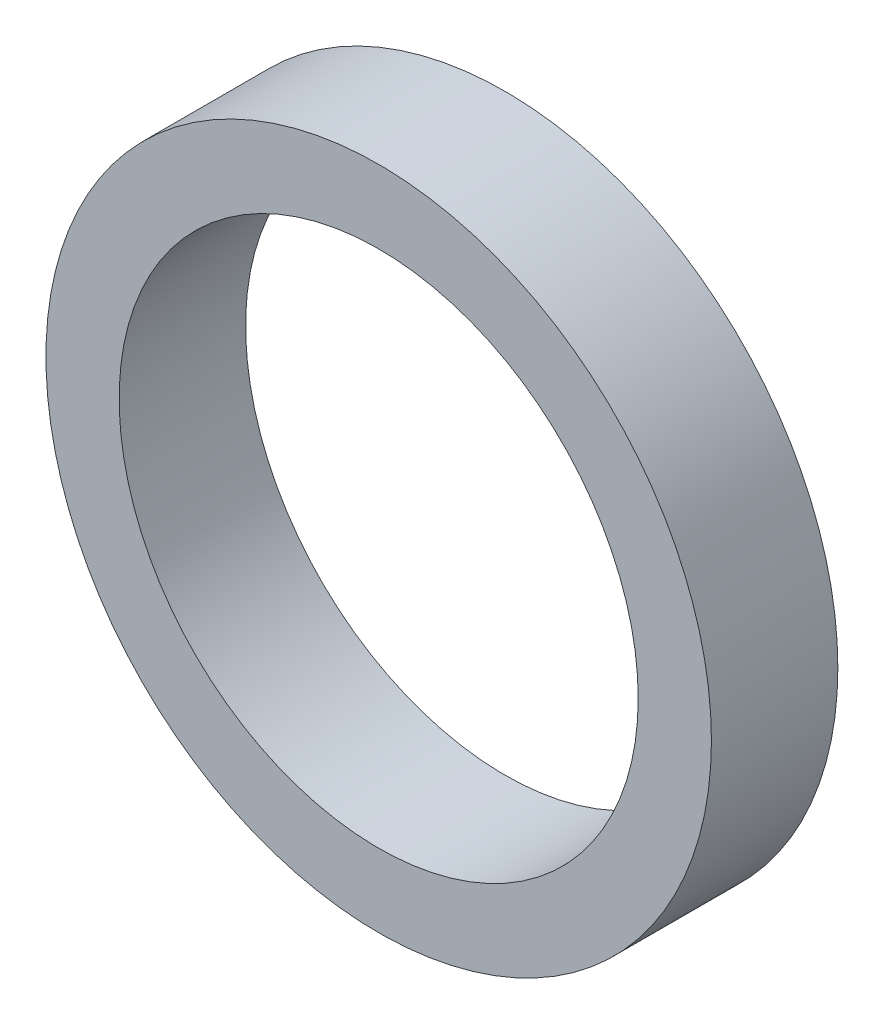
SolidWorks part; units mm, degrees
material "Plain Carbon Steel"
ref_plane "Front Plane" through (0, 0, 0) normal (0, 0, 1) x (1, 0, 0)
ref_plane "Top Plane" through (0, 0, 0) normal (0, 1, 0) x (1, 0, 0)
ref_plane "Right Plane" through (0, 0, 0) normal (1, 0, 0) x (0, 0, -1)
sketch "Bush Ring Profile Ø0.500 x Ø0.390" plane through (0, 0, 0) normal (0, 0, 1) x (1, 0, 0)
  circle A0 centre (0, 0) radius 6.35
  circle A1 centre (0, 0) radius 4.953
  dimension "D1" = 12.7
  dimension "D2" = 9.906
extrude "Bush Ring 0.095 Thick" add sketch "Bush Ring Profile Ø0.500 x Ø0.390" along normal blind 2.413
